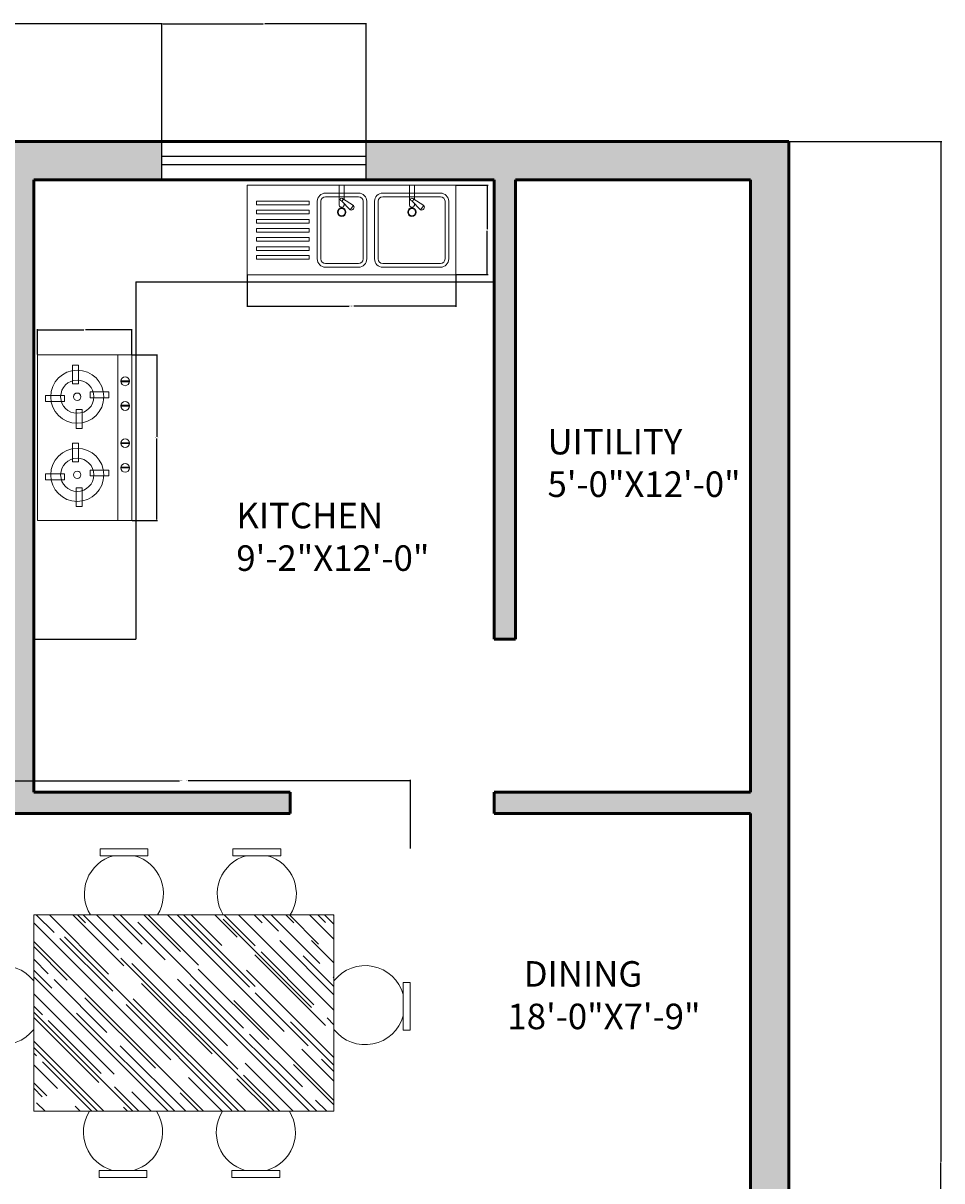
# Model space of a CAD drawing. Units: inches. Extents: x 2831 to 3729, y 3926 to 4974.
# Tile 4 of 8: x 3038 to 3255, y 4702 to 4974. Entities that reach past the tile are written whole.
import ezdxf

# ---------------------------------------------------------------- set-up
doc = ezdxf.new("R2010")
doc.units = ezdxf.units.IN
for name, color, linetype, lineweight in [('A-ANNO-DIMS', 2, 'Continuous', 18), ('A-AREA-IDEN', 7, 'Continuous', 18), ('A-EQPM', 8, 'Continuous', 18), ('A-FLOR-CABN', 8, 'Continuous', 25), ('A-FLOR-FIXT', 9, 'Continuous', 18), ('A-FURN', 8, 'Continuous', 18), ('A-GLAZ', 4, 'Continuous', 25), ('A-WALL', 7, 'Continuous', 50), ('A-WALL-PATT', 252, 'Continuous', 13)]:
    doc.layers.add(name, color=color, linetype=linetype, lineweight=lineweight)
doc.styles.get("Standard").update_dxf_attribs({"font": 'arial.ttf'})
doc.dimstyles.get("Standard").update_dxf_attribs({"dimtxt": 0.18, "dimasz": 0.18, "dimexe": 0.18, "dimexo": 0.0625, "dimgap": 0.09, "dimtad": 0, "dimtih": 1, "dimtoh": 1, "dimdec": 4, "dimzin": 0, "dimdsep": 46, "dimtxsty": 'Standard', "dimcen": 0.09, "dimadec": 0, "dimazin": 0, "dimtfac": 1, "dimtdec": 4, "dimtofl": 0, "dimtmove": 0, "dimatfit": 3, "dimfxl": 1, "dimtolj": 1, "dimtzin": 0, "dimarcsym": 0})

# ---------------------------------------------------------------- blocks, each defined once
blk = doc.blocks.new('A$C6CB038CA')
for p, q in [((0, 0), (0, 488.5)), ((0, 488.5), (1140.7, 488.5)), ((428.4, 445.8), (608.4, 445.8)), ((502.8, 377.5), (502.8, 488.5)), ((529.8, 412.8), (529.8, 488.5)), ((740.8, 445.8), (1055.8, 445.8)), ((886.8, 377.5), (886.8, 488.5)), ((913.8, 412.8), (913.8, 488.5)), ((1140.7, 488.5), (1140.7, 0)), ((52.2, 382.1), (52.2, 402.1)), ((339.4, 402.1), (52.2, 402.1)), ((339.4, 382.1), (52.2, 382.1)), ((339.4, 382.1), (339.4, 402.1)), ((383.4, 85.8), (383.4, 400.8)), ((403.4, 85.8), (403.4, 400.8)), ((428.4, 425.8), (608.4, 425.8)), ((563.7, 353.9), (514.9, 402.4)), ((521.9, 415.4), (580.3, 378.4)), ((529.8, 377.6), (529.8, 387.6)), ((633.4, 85.8), (633.4, 400.8)), ((653.4, 85.8), (653.4, 400.8)), ((695.8, 85.8), (695.8, 400.8)), ((715.8, 85.8), (715.8, 400.8)), ((740.8, 425.8), (1055.8, 425.8)), ((947.8, 353.9), (899, 402.4)), ((906, 415.4), (964.3, 378.4)), ((913.8, 377.6), (913.8, 387.6)), ((1080.8, 85.8), (1080.8, 400.8)), ((1100.8, 85.8), (1100.8, 400.8)), ((52.2, 332.1), (52.2, 352.1)), ((339.4, 352.1), (52.2, 352.1)), ((339.4, 332.1), (52.2, 332.1)), ((339.4, 332.1), (339.4, 352.1)), ((580.3, 378.4), (563.7, 353.9)), ((964.3, 378.4), (947.8, 353.9)), ((52.2, 282.1), (52.2, 302.1)), ((339.4, 302.1), (52.2, 302.1)), ((339.4, 282.1), (52.2, 282.1)), ((339.4, 282.1), (339.4, 302.1)), ((52.2, 232.1), (52.2, 252.1)), ((339.4, 252.1), (52.2, 252.1)), ((339.4, 232.1), (52.2, 232.1)), ((52.2, 182.1), (52.2, 202.1)), ((339.4, 202.1), (52.2, 202.1)), ((339.4, 232.1), (339.4, 252.1)), ((339.4, 182.1), (339.4, 202.1)), ((339.4, 182.1), (52.2, 182.1)), ((52.2, 132.1), (52.2, 152.1)), ((339.4, 152.1), (52.2, 152.1)), ((339.4, 132.1), (52.2, 132.1)), ((339.4, 132.1), (339.4, 152.1)), ((52.2, 84.8), (52.2, 104.8)), ((339.4, 104.8), (52.2, 104.8)), ((339.4, 84.8), (52.2, 84.8)), ((339.4, 84.8), (339.4, 104.8)), ((1140.7, 0), (0, 0)), ((428.4, 60.8), (608.4, 60.8)), ((428.4, 40.8), (608.4, 40.8)), ((740.8, 60.8), (1055.8, 60.8)), ((740.8, 40.8), (1055.8, 40.8))]:
    blk.add_line(p, q)
for centre, radius in [((516.4, 410.5), 7.79), ((900.5, 410.5), 7.79), ((516.9, 341.2), 23.1), ((516.9, 341.3), 19.5), ((900.1, 341.2), 23.1), ((900.2, 341.3), 19.5)]:
    blk.add_circle(centre, radius)
for centre, radius, start, end in [((428.4, 400.8), 45, 90, 180), ((608.4, 400.8), 45, 0, 90), ((740.8, 400.8), 45, 90, 180), ((1055.8, 400.8), 45, 0, 90), ((428.4, 400.8), 25, 90, 180), ((608.4, 400.8), 25, 0, 90), ((740.8, 400.8), 25, 90, 180), ((1055.8, 400.8), 25, 0, 90), ((516.1, 383.8), 14.9, 205.10429, 335.21709), ((568.7, 368.6), 15.5, 251.20242, 39.32146), ((900.1, 383.8), 14.9, 205.10429, 335.21709), ((952.8, 368.6), 15.5, 251.20242, 39.32146), ((428.4, 85.8), 45, 180, 270), ((428.4, 85.8), 25, 180, 270), ((608.4, 85.8), 25, 270, 0), ((608.4, 85.8), 45, 270, 0), ((740.8, 85.8), 45, 180, 270), ((740.8, 85.8), 25, 180, 270), ((1055.8, 85.8), 25, 270, 0), ((1055.8, 85.8), 45, 270, 0)]:
    blk.add_arc(centre, radius, start, end)
blk = doc.blocks.new('A$C67D72025')
at = {"ltscale": 1000}
for p, q in [((385.7, 234.1), (385.7, 209.4)), ((464.6, 234.1), (385.7, 234.1)), ((385.7, 209.4), (464.6, 209.4)), ((464.6, 209.4), (464.6, 234.1)), ((694.4, 59.5), (0, 59.5))]:
    blk.add_line(p, q, dxfattribs=at)
for points in [[(694.4, 396.8), (0, 396.8), (0, 0), (694.4, 0)], [(195.5, 283.6), (195.5, 362.4), (170.8, 362.4), (170.8, 283.6)], [(523.4, 283.6), (523.4, 362.4), (498.6, 362.4), (498.6, 283.6)], [(245, 224.8), (323.9, 224.8), (323.9, 249.5), (245, 249.5)], [(572.8, 224.8), (651.7, 224.8), (651.7, 249.5), (572.8, 249.5)], [(136.8, 234.1), (57.9, 234.1), (57.9, 209.4), (136.8, 209.4)], [(186.3, 175.3), (186.3, 96.5), (211, 96.5), (211, 175.3)], [(514.1, 175.3), (514.1, 96.5), (538.8, 96.5), (538.8, 175.3)], [(223.3, 47.3), (220, 47.3), (220, 9.9), (223.3, 9.9)], [(325.5, 47.3), (322.2, 47.3), (322.2, 9.9), (325.5, 9.9)], [(482.8, 47.3), (479.5, 47.3), (479.5, 9.9), (482.8, 9.9)], [(585, 47.3), (581.6, 47.3), (581.6, 9.9), (585, 9.9)]]:
    blk.add_lwpolyline(points, close=True, dxfattribs=at)
for centre, radius in [((190.9, 229.4), 111.3), ((518.7, 229.4), 111.3), ((190.9, 229.4), 69.6), ((518.7, 229.4), 69.6), ((190.9, 229.4), 15.5), ((518.7, 229.4), 15.5), ((220.3, 28.6), 18.6), ((323.9, 28.6), 18.6), ((480.1, 28.6), 18.6), ((583.7, 28.6), 18.6)]:
    blk.add_circle(centre, radius, dxfattribs=at)
blk = doc.blocks.new('A$C709B6AB6')
for p, q in [((0.969, 1.6731), (0.7259, 1.6731)), ((0.7259, 1.6731), (0.7259, 1.6374)), ((0.969, 1.6374), (0.969, 1.6731)), ((1.6452, 1.6731), (1.402, 1.6731)), ((1.402, 1.6731), (1.402, 1.6374)), ((1.6452, 1.6374), (1.6452, 1.6731)), ((0.7259, 1.6374), (0.969, 1.6374)), ((1.402, 1.6374), (1.6452, 1.6374)), ((0.3883, 0.3366), (0.3883, 1.3366)), ((0.3883, 1.3366), (1.9163, 1.3366)), ((0.4919, 1.2463), (0.4015, 1.3366)), ((0.7693, 1.0352), (0.468, 1.3366)), ((0.8475, 1.0774), (0.5883, 1.3366)), ((0.6526, 1.2956), (0.6117, 1.3366)), ((0.8205, 1.1564), (0.6404, 1.3366)), ((1.3746, 0.6706), (0.7087, 1.3366)), ((0.94, 1.1879), (0.7913, 1.3366)), ((1.0576, 1.108), (0.829, 1.3366)), ((1.4563, 0.7595), (0.9175, 1.2983)), ((1.1357, 1.1502), (0.9493, 1.3366)), ((1.2273, 1.0801), (0.9709, 1.3366)), ((1.6629, 0.7434), (1.0697, 1.3366)), ((1.486, 0.9688), (1.1182, 1.3366)), ((1.5147, 0.9724), (1.1505, 1.3366)), ((1.3459, 1.1807), (1.19, 1.3366)), ((1.424, 1.2229), (1.3103, 1.3366)), ((1.8021, 0.8646), (1.3531, 1.3136)), ((1.5156, 1.178), (1.357, 1.3366)), ((1.9163, 0.8509), (1.4307, 1.3366)), ((1.5506, 1.2956), (1.5097, 1.3366)), ((1.6341, 1.2534), (1.551, 1.3366)), ((1.8443, 1.0882), (1.5959, 1.3366)), ((1.7123, 1.2956), (1.6713, 1.3366)), ((1.838, 1.1879), (1.6893, 1.3366)), ((1.9163, 1.2119), (1.7917, 1.3366)), ((1.8739, 1.2974), (1.8348, 1.3366)), ((1.9163, 1.2891), (1.8689, 1.3366)), ((1.9163, 1.3322), (1.912, 1.3366)), ((1.9163, 0.3366), (1.9163, 1.3366)), ((1.0863, 0.5979), (0.3883, 1.296)), ((1.2525, 0.3366), (0.3883, 1.2008)), ((0.7909, 0.9472), (0.5215, 1.2166)), ((1.4321, 0.3366), (0.5448, 1.2238)), ((1.9163, 0.9299), (1.6404, 1.2058)), ((1.9163, 1.0916), (1.8021, 1.2058)), ((0.5592, 1.0047), (0.3883, 1.1756)), ((1.873, 0.7739), (1.5138, 1.1331)), ((1.8146, 0.879), (1.5452, 1.1484)), ((1.9163, 0.9712), (1.7599, 1.1277)), ((0.4622, 1.037), (0.3883, 1.111)), ((1.6117, 0.3366), (0.8322, 1.116)), ((1.4267, 0.5503), (0.8879, 1.0891)), ((0.4811, 0.9625), (0.3883, 1.0553)), ((1.0729, 0.3366), (0.3883, 1.0212)), ((0.7613, 0.738), (0.4919, 1.0074)), ((1.7913, 0.3366), (1.1196, 1.0083)), ((1.5847, 0.7012), (1.2255, 1.0604)), ((1.9163, 0.6102), (1.4716, 1.055)), ((1.9163, 1.0161), (1.9116, 1.0208)), ((0.0357, 0.9927), (0, 0.9927)), ((0, 0.9927), (0, 0.7495)), ((0.0357, 0.7495), (0.0357, 0.9927)), ((1.2965, 0.6284), (0.9373, 0.9876)), ((1.829, 0.3366), (1.1833, 0.9822)), ((2.269, 0.9927), (2.3047, 0.9927)), ((2.269, 0.7495), (2.269, 0.9927)), ((2.3047, 0.9927), (2.3047, 0.7495)), ((0.7981, 0.5251), (0.3883, 0.935)), ((1.0082, 0.5557), (0.649, 0.9149)), ((1.468, 0.3366), (0.8951, 0.9095)), ((1.9163, 0.3911), (1.4069, 0.9005)), ((1.785, 0.6697), (1.5156, 0.9391)), ((0.4326, 0.8278), (0.3883, 0.8721)), ((0.8933, 0.3366), (0.3883, 0.8416)), ((1.107, 0.3366), (0.6068, 0.8368)), ((1.3971, 0.341), (0.8582, 0.8799)), ((0.7199, 0.4829), (0.3883, 0.8146)), ((0.7316, 0.5287), (0.4622, 0.7981)), ((1.9163, 0.5707), (1.6943, 0.7927)), ((1.9163, 0.7773), (1.882, 0.8116)), ((0, 0.7495), (0.0357, 0.7495)), ((1.7554, 0.4605), (1.486, 0.7299)), ((2.3047, 0.7495), (2.269, 0.7495)), ((0.746, 0.3366), (0.3883, 0.6943)), ((0.7136, 0.3366), (0.3883, 0.662)), ((1.1627, 0.3366), (0.8286, 0.6706)), ((1.9163, 0.4899), (1.7527, 0.6536)), ((0.4029, 0.6185), (0.3883, 0.6332)), ((1.9163, 0.5384), (1.8524, 0.6024)), ((0.5098, 0.4524), (0.3883, 0.5739)), ((0.6849, 0.3366), (0.4326, 0.5889)), ((1.7087, 0.3366), (1.4644, 0.5808)), ((1.9163, 0.3696), (1.7105, 0.5754)), ((0.455, 0.4156), (0.3883, 0.4823)), ((1.3477, 0.3366), (1.1761, 0.5081)), ((1.5883, 0.3366), (1.4222, 0.5027)), ((1.6404, 0.3366), (1.4563, 0.5206)), ((0.4317, 0.4102), (0.3883, 0.4536)), ((0.9238, 0.3366), (0.799, 0.4614)), ((0.9866, 0.3366), (0.8879, 0.4353)), ((1.2273, 0.3366), (1.1339, 0.4299)), ((0.446, 0.3366), (0.4029, 0.3797)), ((0.6256, 0.3366), (0.5996, 0.3626)), ((0.8663, 0.3366), (0.8457, 0.3572)), ((1.8793, 0.3366), (1.8227, 0.3931)), ((1.9163, 0.3366), (0.3883, 0.3366)), ((0.7212, 0), (0.7212, 0.0357)), ((0.7212, 0.0357), (0.9644, 0.0357)), ((0.9644, 0.0357), (0.9644, 0)), ((1.3973, 0), (1.3973, 0.0357)), ((1.3973, 0.0357), (1.6405, 0.0357)), ((1.6405, 0.0357), (1.6405, 0)), ((0.9644, 0), (0.7212, 0)), ((1.6405, 0), (1.3973, 0))]:
    blk.add_line(p, q)
for centre, start, end in [((0.8475, 1.4434), 105.52104, 212.06337), ((0.8475, 1.4434), 327.93663, 74.47896), ((1.5236, 1.4434), 105.52104, 212.06337), ((1.5236, 1.4434), 327.93663, 74.47896), ((0.2296, 0.8768), 37.97614, 164.47896), ((2.075, 0.8768), 15.52104, 142.02386), ((0.2296, 0.8768), 195.52104, 322.02386), ((2.075, 0.8768), 217.97614, 344.47896), ((0.8428, 0.2297), 147.93663, 254.47896), ((0.8428, 0.2297), 285.52104, 32.06337), ((1.5189, 0.2297), 147.93663, 254.47896), ((1.5189, 0.2297), 285.52104, 32.06337)]:
    blk.add_arc(centre, 0.2013, start, end)
blk = doc.blocks.new('*D37')
at = {"layer": 'A-ANNO-DIMS', "color": 0, "lineweight": -2, "transparency": 16777216}
for p, q in [((3091.15, 4914.77), (3091.15, 4907.28)), ((3140.26, 4914.77), (3140.26, 4907.28)), ((3091.33, 4907.46), (3115.16, 4907.46)), ((3140.08, 4907.46), (3116.25, 4907.46))]:
    blk.add_line(p, q, dxfattribs=at)
at = {"layer": 'A-ANNO-DIMS', "color": 0, "transparency": 16777216}
for points in [[(3091.33, 4907.49), (3091.33, 4907.43), (3091.15, 4907.46)], [(3140.08, 4907.49), (3140.08, 4907.43), (3140.26, 4907.46)]]:
    blk.add_solid(points, dxfattribs=at)
at = {"layer": 'Defpoints', "color": 0, "transparency": 16777216}
for p in [(3091.15, 4914.83), (3140.26, 4914.83), (3140.26, 4907.46)]:
    blk.add_point(p, dxfattribs=at)
at = {"layer": 'A-ANNO-DIMS', "color": 0, "transparency": 16777216, "insert": (3115.7, 4907.46), "char_height": 0.18, "attachment_point": 5}
blk.add_mtext('\\A1;SINK 49', dxfattribs=at)
blk = doc.blocks.new('*D38')
at = {"layer": 'A-ANNO-DIMS', "color": 0, "lineweight": -2, "transparency": 16777216}
for p, q in [((3140.32, 4935.86), (3147.81, 4935.86)), ((3147.63, 4935.68), (3147.63, 4925.53)), ((3147.63, 4915.01), (3147.63, 4925.17)), ((3140.32, 4914.83), (3147.81, 4914.83))]:
    blk.add_line(p, q, dxfattribs=at)
at = {"layer": 'A-ANNO-DIMS', "color": 0, "transparency": 16777216}
for points in [[(3147.6, 4935.68), (3147.66, 4935.68), (3147.63, 4935.86)], [(3147.6, 4915.01), (3147.66, 4915.01), (3147.63, 4914.83)]]:
    blk.add_solid(points, dxfattribs=at)
at = {"layer": 'Defpoints', "color": 0, "transparency": 16777216}
for p in [(3140.26, 4935.86), (3147.63, 4935.86), (3140.26, 4914.83)]:
    blk.add_point(p, dxfattribs=at)
at = {"layer": 'A-ANNO-DIMS', "color": 0, "transparency": 16777216, "insert": (3147.63, 4925.35), "char_height": 0.18, "attachment_point": 5}
blk.add_mtext('\\A1;21', dxfattribs=at)
blk = doc.blocks.new('*D39')
at = {"layer": 'A-ANNO-DIMS', "color": 0, "lineweight": -2, "transparency": 16777216}
for p, q in [((3064.14, 4895.98), (3070.09, 4895.98)), ((3069.91, 4895.8), (3069.91, 4876.7)), ((3069.91, 4857.23), (3069.91, 4876.33)), ((3064.14, 4857.05), (3070.09, 4857.05))]:
    blk.add_line(p, q, dxfattribs=at)
at = {"layer": 'A-ANNO-DIMS', "color": 0, "transparency": 16777216}
for points in [[(3069.88, 4895.8), (3069.94, 4895.8), (3069.91, 4895.98)], [(3069.88, 4857.23), (3069.94, 4857.23), (3069.91, 4857.05)]]:
    blk.add_solid(points, dxfattribs=at)
at = {"layer": 'Defpoints', "color": 0, "transparency": 16777216}
for p in [(3064.07, 4895.98), (3069.91, 4895.98), (3064.07, 4857.05)]:
    blk.add_point(p, dxfattribs=at)
at = {"layer": 'A-ANNO-DIMS', "color": 0, "transparency": 16777216, "insert": (3069.91, 4876.51), "char_height": 0.18, "attachment_point": 5}
blk.add_mtext('\\A1;HOB 39', dxfattribs=at)
blk = doc.blocks.new('*D40')
at = {"layer": 'A-ANNO-DIMS', "color": 0, "lineweight": -2, "transparency": 16777216}
for p, q in [((3041.83, 4896.04), (3041.83, 4902)), ((3042.01, 4901.82), (3052.73, 4901.82)), ((3063.89, 4901.82), (3053.17, 4901.82)), ((3064.07, 4896.04), (3064.07, 4902))]:
    blk.add_line(p, q, dxfattribs=at)
at = {"layer": 'A-ANNO-DIMS', "color": 0, "transparency": 16777216}
for points in [[(3042.01, 4901.85), (3042.01, 4901.79), (3041.83, 4901.82)], [(3063.89, 4901.85), (3063.89, 4901.79), (3064.07, 4901.82)]]:
    blk.add_solid(points, dxfattribs=at)
at = {"layer": 'Defpoints', "color": 0, "transparency": 16777216}
for p in [(3041.83, 4901.82), (3041.83, 4895.98), (3064.07, 4895.98)]:
    blk.add_point(p, dxfattribs=at)
at = {"layer": 'A-ANNO-DIMS', "color": 0, "transparency": 16777216, "insert": (3052.95, 4901.82), "char_height": 0.18, "attachment_point": 5}
blk.add_mtext('\\A1;22', dxfattribs=at)
blk = doc.blocks.new('*D41')
at = {"layer": 'A-ANNO-DIMS', "color": 0, "lineweight": -2, "transparency": 16777216}
for p, q in [((3023.02, 4779.92), (3023.02, 4796.01)), ((3023.2, 4795.83), (3075.24, 4795.83)), ((3129.35, 4795.83), (3077.31, 4795.83)), ((3129.53, 4779.92), (3129.53, 4796.01))]:
    blk.add_line(p, q, dxfattribs=at)
at = {"layer": 'A-ANNO-DIMS', "color": 0, "transparency": 16777216}
for points in [[(3023.2, 4795.86), (3023.2, 4795.8), (3023.02, 4795.83)], [(3129.35, 4795.86), (3129.35, 4795.8), (3129.53, 4795.83)]]:
    blk.add_solid(points, dxfattribs=at)
at = {"layer": 'Defpoints', "color": 0, "transparency": 16777216}
for p in [(3129.53, 4795.83), (3023.02, 4779.86), (3129.53, 4779.86)]:
    blk.add_point(p, dxfattribs=at)
at = {"layer": 'A-ANNO-DIMS', "color": 0, "transparency": 16777216, "insert": (3076.27, 4795.83), "char_height": 0.18, "attachment_point": 5}
blk.add_mtext('\\A1;DINING SET 107', dxfattribs=at)
blk = doc.blocks.new('*D48')
at = {"layer": 'A-ANNO-DIMS', "color": 0, "lineweight": -2, "transparency": 16777216}
for p, q in [((3218.55, 4946.14), (3254.48, 4946.14)), ((3254.3, 4945.96), (3254.3, 4706.32)), ((3254.3, 4466.32), (3254.3, 4705.96)), ((3218.55, 4466.14), (3254.48, 4466.14))]:
    blk.add_line(p, q, dxfattribs=at)
at = {"layer": 'A-ANNO-DIMS', "color": 0, "transparency": 16777216}
for points in [[(3254.27, 4945.96), (3254.33, 4945.96), (3254.3, 4946.14)], [(3254.27, 4466.32), (3254.33, 4466.32), (3254.3, 4466.14)]]:
    blk.add_solid(points, dxfattribs=at)
at = {"layer": 'Defpoints', "color": 0, "transparency": 16777216}
for p in [(3218.49, 4946.14), (3254.3, 4946.14), (3218.49, 4466.14)]:
    blk.add_point(p, dxfattribs=at)
at = {"layer": 'A-ANNO-DIMS', "color": 0, "transparency": 16777216, "insert": (3254.3, 4706.14), "char_height": 0.18, "attachment_point": 5}
blk.add_mtext('\\A1;480', dxfattribs=at)
blk = doc.blocks.new('*D52')
at = {"layer": 'A-ANNO-DIMS', "color": 0, "lineweight": -2, "transparency": 16777216}
for p, q in [((2987.74, 4946.2), (2987.74, 4973.97)), ((2987.92, 4973.79), (3029.03, 4973.79)), ((3070.94, 4973.79), (3029.82, 4973.79)), ((3071.12, 4946.2), (3071.12, 4973.97))]:
    blk.add_line(p, q, dxfattribs=at)
at = {"layer": 'A-ANNO-DIMS', "color": 0, "transparency": 16777216}
for points in [[(2987.92, 4973.82), (2987.92, 4973.76), (2987.74, 4973.79)], [(3070.94, 4973.82), (3070.94, 4973.76), (3071.12, 4973.79)]]:
    blk.add_solid(points, dxfattribs=at)
at = {"layer": 'Defpoints', "color": 0, "transparency": 16777216}
for p in [(3071.12, 4973.79), (2987.74, 4946.14), (3071.12, 4946.14)]:
    blk.add_point(p, dxfattribs=at)
at = {"layer": 'A-ANNO-DIMS', "color": 0, "transparency": 16777216, "insert": (3029.43, 4973.79), "char_height": 0.18, "attachment_point": 5}
blk.add_mtext('\\A1;83.38', dxfattribs=at)
blk = doc.blocks.new('*D53')
at = {"layer": 'A-ANNO-DIMS', "color": 0, "lineweight": -2, "transparency": 16777216}
for p, q in [((3071.12, 4946.2), (3071.12, 4973.97)), ((3071.3, 4973.79), (3094.89, 4973.79)), ((3118.94, 4973.79), (3095.34, 4973.79)), ((3119.12, 4946.2), (3119.12, 4973.97))]:
    blk.add_line(p, q, dxfattribs=at)
at = {"layer": 'A-ANNO-DIMS', "color": 0, "transparency": 16777216}
for points in [[(3071.3, 4973.82), (3071.3, 4973.76), (3071.12, 4973.79)], [(3118.94, 4973.82), (3118.94, 4973.76), (3119.12, 4973.79)]]:
    blk.add_solid(points, dxfattribs=at)
at = {"layer": 'Defpoints', "color": 0, "transparency": 16777216}
for p in [(3119.12, 4973.79), (3071.12, 4946.14), (3119.12, 4946.14)]:
    blk.add_point(p, dxfattribs=at)
at = {"layer": 'A-ANNO-DIMS', "color": 0, "transparency": 16777216, "insert": (3095.12, 4973.79), "char_height": 0.18, "attachment_point": 5}
blk.add_mtext('\\A1;48', dxfattribs=at)

msp = doc.modelspace()

# ---------------------------------------------------------------- hatches: boundary and pattern name
at = {"layer": 'A-WALL-PATT'}
h = msp.add_hatch(color=256, dxfattribs=at)
h.dxf.hatch_style = 1
h.paths.add_polyline_path([(2867.4912, 4707.1405), (2999.9912, 4707.1405), (2999.9912, 4712.1405), (2867.4912, 4712.1405), (2867.4912, 4788.1405), (2999.9912, 4788.1405), (2999.9912, 4793.1405), (2867.4912, 4793.1405), (2867.4912, 4937.1405), (2915.7412, 4937.1405), (2915.7412, 4946.1405), (2858.4912, 4946.1405), (2858.4912, 4526.1405), (2895.7412, 4526.1405), (2895.7412, 4535.1405), (2867.4912, 4535.1405)])
h.paths.add_polyline_path([(3071.1162, 4946.1405), (2987.7412, 4946.1405), (2987.7412, 4937.1405), (3035.9912, 4937.1405), (3035.9912, 4788.1405), (3101.2412, 4788.1405), (3101.2412, 4793.1405), (3040.9912, 4793.1405), (3040.9912, 4937.1405), (3071.1162, 4937.1405)])
h = msp.add_hatch(color=256, dxfattribs=at)
h.dxf.hatch_style = 1
h.paths.add_polyline_path([(3218.4912, 4946.1405), (3119.1162, 4946.1405), (3119.1162, 4937.1405), (3149.2412, 4937.1405), (3149.2412, 4829.1405), (3154.2412, 4829.1405), (3154.2412, 4937.1405), (3209.4912, 4937.1405), (3209.4912, 4793.1405), (3149.2412, 4793.1405), (3149.2412, 4788.1405), (3209.4912, 4788.1405), (3209.4912, 4695.1405), (3120.4912, 4695.1405), (3120.4912, 4666.1405), (3125.4912, 4666.1405), (3125.4912, 4690.1405), (3209.4912, 4690.1405), (3209.4912, 4675.1405), (3218.4912, 4675.1405)])

# ---------------------------------------------------------------- linework, layer by layer
at = {"layer": 'A-FLOR-CABN'}
for p, q in [((3064.9912, 4913.1405), (3149.2412, 4913.1405)), ((3064.9912, 4913.1405), (3064.9912, 4829.1405)), ((3040.9912, 4829.1405), (3064.9912, 4829.1405))]:
    msp.add_line(p, q, dxfattribs=at)
at = {"layer": 'A-GLAZ'}
for p, q in [((3071.1162, 4937.1405), (3071.1162, 4946.1405)), ((3119.1162, 4937.1405), (3119.1162, 4946.1405)), ((3119.1162, 4942.6405), (3071.1162, 4942.6405)), ((3119.1162, 4940.6405), (3071.1162, 4940.6405))]:
    msp.add_line(p, q, dxfattribs=at)
at = {"layer": 'A-WALL'}
for p, q in [((2858.4912, 4946.1405), (3218.4912, 4946.1405)), ((3218.4912, 4946.1405), (3218.4912, 4466.1405)), ((3040.9912, 4937.1405), (3149.2412, 4937.1405)), ((3040.9912, 4937.1405), (3040.9912, 4793.1405)), ((3149.2412, 4937.1405), (3149.2412, 4829.1405)), ((3154.2412, 4937.1405), (3154.2412, 4829.1405)), ((3154.2412, 4937.1405), (3209.4912, 4937.1405)), ((3209.4912, 4937.1405), (3209.4912, 4793.1405)), ((3149.2412, 4829.1405), (3154.2412, 4829.1405)), ((3040.9912, 4793.1405), (3101.2412, 4793.1405)), ((3101.2412, 4793.1405), (3101.2412, 4788.1405)), ((3149.2412, 4793.1405), (3209.4912, 4793.1405)), ((3149.2412, 4793.1405), (3149.2412, 4788.1405)), ((3035.9912, 4788.1405), (3101.2412, 4788.1405)), ((3149.2412, 4788.1405), (3209.4912, 4788.1405)), ((3209.4912, 4788.1405), (3209.4912, 4695.1405))]:
    msp.add_line(p, q, dxfattribs=at)

# ---------------------------------------------------------------- block references
at = {"layer": 'A-EQPM', "xscale": 0.0560624064263751, "yscale": 0.0560624064263751, "zscale": 0.0560624064263751, "rotation": 90}
msp.add_blockref('A$C67D72025', (3064.0735, 4857.047), dxfattribs=at)
at = {"layer": 'A-FLOR-FIXT', "xscale": 0.0430565998065705, "yscale": 0.0430565998065705, "zscale": 0.0430565998065705}
msp.add_blockref('A$C6CB038CA', (3091.1466, 4914.8282), dxfattribs=at)
at = {"layer": 'A-FURN', "xscale": 46.21065113701777, "yscale": 46.21065113701777, "zscale": 46.21065113701777}
msp.add_blockref('A$C709B6AB6', (3023.0222, 4702.5423), dxfattribs=at)

# ---------------------------------------------------------------- texts
at = {"layer": 'A-AREA-IDEN', "attachment_point": 1}
for s, width, insert, char_height in [('UITILITY\\P5\'-0"X12\'-0"', 40.448371, (3161.7821, 4878.5612), 6), ('KITCHEN\\P9\'-2"X12\'-0"', 48.741532, (3088.614, 4861.1834), 6), ('     {\\H2.4x;DINING\\P18\'-0"X7\'-9"}', 48.741532, (3152.3592, 4753.4073), 2.5)]:
    msp.add_mtext_dynamic_manual_height_columns(s, width=width, gutter_width=12.5, heights=[0], dxfattribs=dict(at, insert=insert, char_height=char_height))

# ---------------------------------------------------------------- dimensions: what is measured, and where the dimension line sits
at = {"layer": 'A-ANNO-DIMS'}
for base, p1, p2, override, picture, middle in [((3071.116169, 4973.790495), (2987.741169, 4946.140495), (3071.116169, 4946.140495), {"dimdec": 2, "dimlfac": 1, "dimrnd": 0, "dimzin": 0, "dimdsep": 46, "dimlunit": 2}, '*D52', (3029.428669, 4973.790495)), ((3119.1162, 4973.7905), (3071.1162, 4946.1405), (3119.1162, 4946.1405), {"dimdec": 0, "dimlfac": 1, "dimrnd": 0, "dimzin": 0, "dimdsep": 46, "dimlunit": 2}, '*D53', (3095.1162, 4973.7905))]:
    dim = msp.add_linear_dim(base=base, p1=p1, p2=p2, dimstyle='Standard', override=override, dxfattribs=at)
    dim.commit()
    dim.dimension.update_dxf_attribs({"geometry": picture, "text_midpoint": middle})
for base, p1, p2, angle, picture, middle in [((3254.2994, 4946.1405), (3218.4912, 4466.1405), (3218.4912, 4946.1405), 90, '*D48', (3254.2994, 4706.1405)), ((3147.6274, 4935.8627), (3140.2603, 4914.8282), (3140.2603, 4935.8627), 90, '*D38', (3147.6274, 4925.3454)), ((3041.8274, 4901.8172), (3064.0735, 4895.9776), (3041.8274, 4895.9776), 180, '*D40', (3052.9505, 4901.8172))]:
    dim = msp.add_linear_dim(base=base, p1=p1, p2=p2, angle=angle, dimstyle='Standard', override={"dimdec": 0, "dimlfac": 1, "dimrnd": 0, "dimzin": 0, "dimdsep": 46, "dimlunit": 2}, dxfattribs=at)
    dim.commit()
    dim.dimension.update_dxf_attribs({"geometry": picture, "text_midpoint": middle})
for base, p1, p2, text, picture, middle in [((3140.2603, 4907.4611), (3091.1466, 4914.8282), (3140.2603, 4914.8282), 'SINK <>', '*D37', (3115.7035, 4907.4611)), ((3129.5255, 4795.8345), (3023.0222, 4779.8591), (3129.5255, 4779.8591), 'DINING SET <>', '*D41', (3076.2739, 4795.8345))]:
    dim = msp.add_linear_dim(base=base, p1=p1, p2=p2, text=text, dimstyle='Standard', override={"dimdec": 0, "dimlfac": 1, "dimrnd": 0, "dimzin": 0, "dimdsep": 46, "dimlunit": 2}, dxfattribs=at)
    dim.commit()
    dim.dimension.update_dxf_attribs({"geometry": picture, "text_midpoint": middle})
dim = msp.add_linear_dim(base=(3069.9131, 4895.9776), p1=(3064.0735, 4857.047), p2=(3064.0735, 4895.9776), angle=90, text='HOB <>', dimstyle='Standard', override={"dimdec": 0, "dimlfac": 1, "dimrnd": 0, "dimzin": 0, "dimdsep": 46, "dimlunit": 2}, dxfattribs=at)
dim.commit()
dim.dimension.update_dxf_attribs({"geometry": '*D39', "text_midpoint": (3069.9131, 4876.5123)})

doc.saveas('drawing.dxf')
